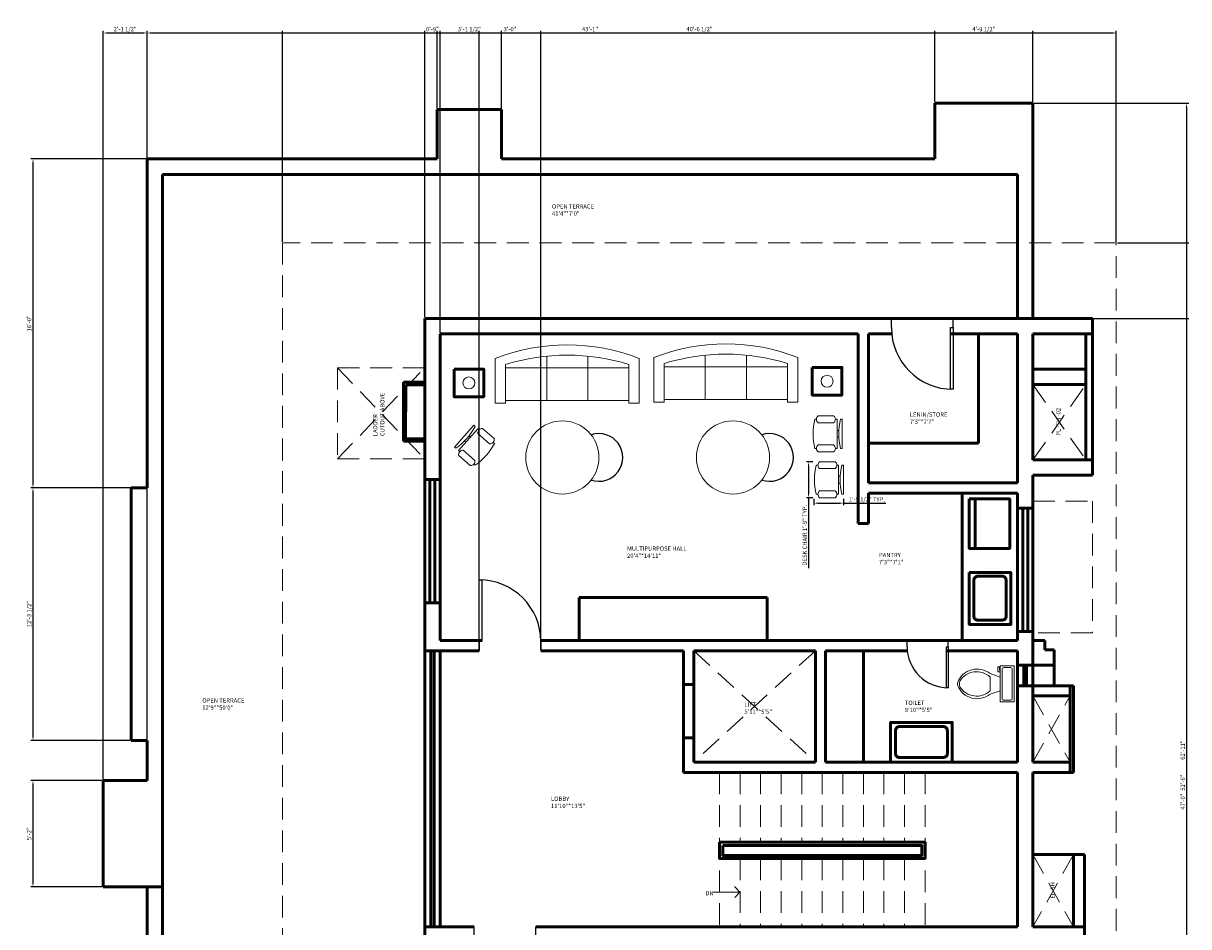
# Model space of a CAD drawing. Units: inches. Extents: x 5312 to 23584, y 2846 to 7447.
# Tile 8 of 12: x 10620 to 11300, y 3352 to 3879. Entities that reach past the tile are written whole.
import ezdxf

# ---------------------------------------------------------------- set-up
doc = ezdxf.new("R2010")
doc.units = ezdxf.units.IN
doc.linetypes.add('DASHED', pattern=[19.05, 12.7, -6.35])
for name, color, linetype, lineweight in [('A-ANNO-DIMS', 2, 'Continuous', 18), ('A-ANNO-TEXT', 3, 'Continuous', 18), ('A-AREA-IDEN', 7, 'Continuous', 18), ('A-DOOR', 4, 'Continuous', 25), ('A-FLOR-FIXT', 9, 'Continuous', 18), ('A-FLOR-OVHD', 8, 'DASHED', 18), ('A-FLOR-STRS', 3, 'Continuous', 18), ('A-FURN', 8, 'Continuous', 18), ('A-WALL', 7, 'Continuous', 50)]:
    doc.layers.add(name, color=color, linetype=linetype, lineweight=lineweight)
doc.styles.get("Standard").update_dxf_attribs({"font": 'arial.ttf'})
doc.dimstyles.new('ISO-25', dxfattribs={"dimtxt": 2.5, "dimasz": 2.5, "dimexe": 1.25, "dimexo": 0.625, "dimtad": 1, "dimlunit": 3, "dimtxsty": 'Standard', "dimcen": 2.5, "dimadec": 0, "dimazin": 0, "dimtfac": 1, "dimtmove": 0, "dimatfit": 3, "dimfxl": 1, "dimarcsym": 0})

# ---------------------------------------------------------------- blocks, each defined once
blk = doc.blocks.new('*U2')
for p, q in [((0, 0), (0, -6)), ((40, 0), (40, -6))]:
    blk.add_line(p, q)
blk.add_lwpolyline([(0, 0), (0, 40), (1.75, 40), (1.75, 0)], close=True)
blk.add_arc((0, 0), 40, 0, 90)
blk = doc.blocks.new('Sofa - Roundback 7 ft.')
for p, q in [((-12.00002, -32.4421), (-12.00003, -6.5971)), ((11.99997, -32.4421), (11.99998, -6.5971)), ((-36.000027, -34), (-36.000027, -11.4696)), ((-35.999844, -13.3819), (35.9998, -13.3819)), ((35.99998, -34), (35.99998, -11.4696)), ((-36.000027, -32.4421), (35.99998, -32.4421))]:
    blk.add_line(p, q)
for points in [[(-36.000027, -34), (-42.000027, -34), (-42.000027, -8)], [(41.99998, -8), (41.99998, -34), (35.99998, -34)]]:
    blk.add_lwpolyline(points)
for centre, radius, start, end in [((0, -114.25), 114.25, 68.43141, 111.5686), ((-0.00001, -127.1968), 121.1968, 72.72033, 107.2797)]:
    blk.add_arc(centre, radius, start, end)
blk = doc.blocks.new('Chair - Desk')
for p, q in [((-8.5, 0), (-8.5, -1)), ((-8.5, 0), (8.5, 0)), ((8.5, 0), (8.5, -1)), ((-10.5, -5), (-10.5, -14)), ((-8.5, -3), (-8.5, -4)), ((-8.5, -3), (8.5, -3)), ((-6.5, -14), (-6.5, -5)), ((-2, -3), (-2, -1.9355)), ((2, -1.9576), (2, -3)), ((6.5, -5), (6.5, -14)), ((8.5, -3), (8.5, -4)), ((10.5, -14), (10.5, -5)), ((-8.5, -15), (-8.5, -16)), ((8.5, -15), (8.5, -16))]:
    blk.add_line(p, q)
for centre, radius, start, end in [((-8.5, -6.5), 2.5, 36.8699, 143.1301), ((0, 34.625), 36.625, 256.5803, 283.4197), ((8.5, -6.5), 2.5, 36.8699, 143.1301), ((-8.5, -12.5), 2.5, 216.8699, 323.1301), ((0, 19.625), 36.625, 256.5803, 283.4197), ((8.5, -12.5), 2.5, 216.8699, 323.1301)]:
    blk.add_arc(centre, radius, start, end)
blk = doc.blocks.new('Toilet - top')
for p, q in [((9.5, -6), (9.5, -2)), ((-10, -8.5), (-8, -8.5)), ((-10, -9.5), (-10, -8.5)), ((-7, -9.5), (-10, -9.5)), ((-8, -8.5), (-8, -8)), ((-7, -8), (-7, -9.5)), ((-4, -8), (-6, -14)), ((4, -8), (6, -14)), ((4, -14), (-4, -14))]:
    blk.add_line(p, q)
blk.add_lwpolyline([(10.5, -8), (10.5, 0), (-10.5, 0), (-10.5, -8)], close=True)
for points in [[(-9.5, -2), (-9.5, -6)], [(8.5, -1), (-8.5, -1)], [(-8.5, -7), (8.5, -7)]]:
    blk.add_lwpolyline(points)
for centre, radius, start, end in [((-8.62, -1.88), 0.884, 81.8699, 188.1301), ((-8.62, -6.12), 0.884, 171.8699, 278.1301), ((8.62, -1.88), 0.884, 351.8699, 98.1301), ((8.62, -6.12), 0.884, 261.8699, 8.1301), ((3.52, -21.58), 12.17, 141.46911, 247.97143), ((4.2, -21.82), 11.33, 136.36773, 238.94682), ((-3.52, -21.58), 12.17, 292.02843, 38.53071), ((-4.2, -21.82), 11.33, 301.05301, 43.63209), ((0, -27.88), 4, 245.73182, 294.26817), ((0, -29), 4, 254.86053, 285.13947)]:
    blk.add_arc(centre, radius, start, end)
blk = doc.blocks.new('STAIR-ARROW')
for p, q in [((0, 3.17), (16.03, 3.17)), ((16.03, 3.17), (12.89, 6.38)), ((16.03, 3.17), (13.15, 0))]:
    blk.add_line(p, q)
blk = doc.blocks.new('*D31')
at = {"layer": 'A-ANNO-DIMS', "color": 0, "lineweight": -2, "transparency": 16777216}
for p, q in [((11080.5, 3623.27), (11076.72, 3623.27)), ((11077.97, 3620.77), (11077.97, 3604.77)), ((11080.5, 3602.27), (11076.72, 3602.27)), ((11077.97, 3602.27), (11077.97, 3561.09))]:
    blk.add_line(p, q, dxfattribs=at)
at = {"layer": 'A-ANNO-DIMS', "color": 0, "transparency": 16777216}
for points in [[(11077.56, 3620.77), (11078.39, 3620.77), (11077.97, 3623.27)], [(11077.56, 3604.77), (11078.39, 3604.77), (11077.97, 3602.27)]]:
    blk.add_solid(points, dxfattribs=at)
at = {"layer": 'DEFPOINTS', "color": 0, "transparency": 16777216}
for p in [(11081.12, 3623.27), (11077.97, 3602.27), (11081.12, 3602.27)]:
    blk.add_point(p, dxfattribs=at)
at = {"layer": 'A-ANNO-DIMS', "color": 0, "transparency": 16777216, "insert": (11076.06, 3580.43), "char_height": 2.5, "attachment_point": 5, "rotation": 90}
blk.add_mtext('DESK CHAIR 1\'-9" TYP.', dxfattribs=at)
blk = doc.blocks.new('*D32')
at = {"layer": 'A-ANNO-DIMS', "color": 0, "lineweight": -2, "transparency": 16777216}
for p, q in [((11081.12, 3601.65), (11081.12, 3597.87)), ((11083.62, 3599.12), (11095.96, 3599.12)), ((11098.46, 3601.65), (11098.46, 3597.87)), ((11098.46, 3599.12), (11123.04, 3599.12))]:
    blk.add_line(p, q, dxfattribs=at)
at = {"layer": 'A-ANNO-DIMS', "color": 0, "transparency": 16777216}
for points in [[(11083.62, 3599.54), (11083.62, 3598.71), (11081.12, 3599.12)], [(11095.96, 3599.54), (11095.96, 3598.71), (11098.46, 3599.12)]]:
    blk.add_solid(points, dxfattribs=at)
at = {"layer": 'DEFPOINTS', "color": 0, "transparency": 16777216}
for p in [(11081.12, 3602.27), (11098.46, 3602.27), (11098.46, 3599.12)]:
    blk.add_point(p, dxfattribs=at)
at = {"layer": 'A-ANNO-DIMS', "color": 0, "transparency": 16777216, "insert": (11112, 3601.04), "char_height": 2.5, "attachment_point": 5}
blk.add_mtext('1\'-5 1/2" TYP.', dxfattribs=at)
blk = doc.blocks.new('*D83')
at = {"layer": 'A-ANNO-DIMS', "color": 0, "lineweight": -2, "transparency": 16777216}
for p, q in [((10691.96, 3800.6), (10691.96, 3874.73)), ((10694.46, 3873.48), (11206.46, 3873.48)), ((11208.96, 3800.6), (11208.96, 3874.73))]:
    blk.add_line(p, q, dxfattribs=at)
at = {"layer": 'A-ANNO-DIMS', "color": 0, "transparency": 16777216}
for points in [[(10694.46, 3873.9), (10694.46, 3873.07), (10691.96, 3873.48)], [(11206.46, 3873.9), (11206.46, 3873.07), (11208.96, 3873.48)]]:
    blk.add_solid(points, dxfattribs=at)
at = {"layer": 'DEFPOINTS', "color": 0, "transparency": 16777216}
for p in [(11208.96, 3873.48), (10691.96, 3799.97), (11208.96, 3799.97)]:
    blk.add_point(p, dxfattribs=at)
at = {"layer": 'A-ANNO-DIMS', "color": 0, "transparency": 16777216, "insert": (10950.46, 3875.39), "char_height": 2.5, "attachment_point": 5}
blk.add_mtext('43\'-1"', dxfattribs=at)
blk = doc.blocks.new('*D84')
at = {"layer": 'A-ANNO-DIMS', "color": 0, "lineweight": -2, "transparency": 16777216}
for p, q in [((11209.58, 3832.48), (11299.83, 3832.48)), ((11298.58, 3829.98), (11298.58, 3080.08)), ((11209.58, 3077.58), (11299.83, 3077.58))]:
    blk.add_line(p, q, dxfattribs=at)
at = {"layer": 'A-ANNO-DIMS', "color": 0, "transparency": 16777216}
for points in [[(11298.16, 3829.98), (11298.99, 3829.98), (11298.58, 3832.48)], [(11298.16, 3080.08), (11298.99, 3080.08), (11298.58, 3077.58)]]:
    blk.add_solid(points, dxfattribs=at)
at = {"layer": 'DEFPOINTS', "color": 0, "transparency": 16777216}
for p in [(11208.96, 3832.48), (11208.96, 3077.58), (11298.58, 3077.58)]:
    blk.add_point(p, dxfattribs=at)
at = {"layer": 'A-ANNO-DIMS', "color": 0, "transparency": 16777216, "insert": (11296.68, 3455.03), "char_height": 2.5, "attachment_point": 5, "rotation": 90}
blk.add_mtext('62\'-11"', dxfattribs=at)
blk = doc.blocks.new('*D85')
at = {"layer": 'A-ANNO-DIMS', "color": 0, "lineweight": -2, "transparency": 16777216}
for p, q in [((10666.36, 3437.87), (10666.36, 3874.73)), ((10668.86, 3873.48), (10689.46, 3873.48)), ((10691.96, 3461.27), (10691.96, 3874.73))]:
    blk.add_line(p, q, dxfattribs=at)
at = {"layer": 'A-ANNO-DIMS', "color": 0, "transparency": 16777216}
for points in [[(10668.86, 3873.9), (10668.86, 3873.07), (10666.36, 3873.48)], [(10689.46, 3873.9), (10689.46, 3873.07), (10691.96, 3873.48)]]:
    blk.add_solid(points, dxfattribs=at)
at = {"layer": 'DEFPOINTS', "color": 0, "transparency": 16777216}
for p in [(10691.96, 3873.48), (10691.96, 3460.64), (10666.36, 3437.25)]:
    blk.add_point(p, dxfattribs=at)
at = {"layer": 'A-ANNO-DIMS', "color": 0, "transparency": 16777216, "insert": (10679.16, 3875.4), "char_height": 2.5, "attachment_point": 5}
blk.add_mtext('2\'-1 1/2"', dxfattribs=at)
blk = doc.blocks.new('*D86')
at = {"layer": 'A-ANNO-DIMS', "color": 0, "lineweight": -2, "transparency": 16777216}
for p, q in [((10691.33, 3799.97), (10624.11, 3799.97)), ((10625.36, 3797.47), (10625.36, 3610.55)), ((10691.33, 3608.05), (10624.11, 3608.05))]:
    blk.add_line(p, q, dxfattribs=at)
at = {"layer": 'A-ANNO-DIMS', "color": 0, "transparency": 16777216}
for points in [[(10624.94, 3797.47), (10625.78, 3797.47), (10625.36, 3799.97)], [(10624.94, 3610.55), (10625.78, 3610.55), (10625.36, 3608.05)]]:
    blk.add_solid(points, dxfattribs=at)
at = {"layer": 'DEFPOINTS', "color": 0, "transparency": 16777216}
for p in [(10691.96, 3799.97), (10625.36, 3608.05), (10691.96, 3608.05)]:
    blk.add_point(p, dxfattribs=at)
at = {"layer": 'A-ANNO-DIMS', "color": 0, "transparency": 16777216, "insert": (10623.46, 3704.01), "char_height": 2.5, "attachment_point": 5, "rotation": 90}
blk.add_mtext('16\'-0"', dxfattribs=at)
blk = doc.blocks.new('*D87')
at = {"layer": 'A-ANNO-DIMS', "color": 0, "lineweight": -2, "transparency": 16777216}
for p, q in [((10682.12, 3608.05), (10624.11, 3608.05)), ((10625.36, 3605.55), (10625.36, 3463.14)), ((10682.12, 3460.64), (10624.11, 3460.64))]:
    blk.add_line(p, q, dxfattribs=at)
at = {"layer": 'A-ANNO-DIMS', "color": 0, "transparency": 16777216}
for points in [[(10624.94, 3605.55), (10625.78, 3605.55), (10625.36, 3608.05)], [(10624.94, 3463.14), (10625.78, 3463.14), (10625.36, 3460.64)]]:
    blk.add_solid(points, dxfattribs=at)
at = {"layer": 'DEFPOINTS', "color": 0, "transparency": 16777216}
for p in [(10682.74, 3608.05), (10625.36, 3460.64), (10682.74, 3460.64)]:
    blk.add_point(p, dxfattribs=at)
at = {"layer": 'A-ANNO-DIMS', "color": 0, "transparency": 16777216, "insert": (10623.44, 3534.35), "char_height": 2.5, "attachment_point": 5, "rotation": 90}
blk.add_mtext('12\'-3 1/2"', dxfattribs=at)
blk = doc.blocks.new('*D88')
at = {"layer": 'A-ANNO-DIMS', "color": 0, "lineweight": -2, "transparency": 16777216}
for p, q in [((10665.73, 3437.25), (10624.11, 3437.25)), ((10625.36, 3434.75), (10625.36, 3377.7)), ((10665.73, 3375.2), (10624.11, 3375.2))]:
    blk.add_line(p, q, dxfattribs=at)
at = {"layer": 'A-ANNO-DIMS', "color": 0, "transparency": 16777216}
for points in [[(10624.94, 3434.75), (10625.78, 3434.75), (10625.36, 3437.25)], [(10624.94, 3377.7), (10625.78, 3377.7), (10625.36, 3375.2)]]:
    blk.add_solid(points, dxfattribs=at)
at = {"layer": 'DEFPOINTS', "color": 0, "transparency": 16777216}
for p in [(10666.36, 3437.25), (10625.36, 3375.2), (10666.36, 3375.2)]:
    blk.add_point(p, dxfattribs=at)
at = {"layer": 'A-ANNO-DIMS', "color": 0, "transparency": 16777216, "insert": (10623.46, 3406.22), "char_height": 2.5, "attachment_point": 5, "rotation": 90}
blk.add_mtext('5\'-2"', dxfattribs=at)
blk = doc.blocks.new('*D91')
at = {"layer": 'A-ANNO-DIMS', "color": 0, "lineweight": -2, "transparency": 16777216}
for p, q in [((11200.58, 3706.97), (11299.83, 3706.97)), ((11298.58, 3704.47), (11298.58, 3145.47)), ((11200.58, 3142.97), (11299.83, 3142.97))]:
    blk.add_line(p, q, dxfattribs=at)
at = {"layer": 'A-ANNO-DIMS', "color": 0, "transparency": 16777216}
for points in [[(11298.16, 3704.47), (11298.99, 3704.47), (11298.58, 3706.97)], [(11298.16, 3145.47), (11298.99, 3145.47), (11298.58, 3142.97)]]:
    blk.add_solid(points, dxfattribs=at)
at = {"layer": 'DEFPOINTS', "color": 0, "transparency": 16777216}
for p in [(11199.96, 3706.97), (11199.96, 3142.97), (11298.58, 3142.97)]:
    blk.add_point(p, dxfattribs=at)
at = {"layer": 'A-ANNO-DIMS', "color": 0, "transparency": 16777216, "insert": (11296.68, 3424.97), "char_height": 2.5, "attachment_point": 5, "rotation": 90}
blk.add_mtext('47\'-0"', dxfattribs=at)
blk = doc.blocks.new('*D92')
at = {"layer": 'A-ANNO-DIMS', "color": 0, "lineweight": -2, "transparency": 16777216}
for p, q in [((10861.16, 3829.39), (10861.16, 3874.73)), ((10863.66, 3873.48), (10896.32, 3873.48)), ((10898.82, 3829.39), (10898.82, 3874.73))]:
    blk.add_line(p, q, dxfattribs=at)
at = {"layer": 'A-ANNO-DIMS', "color": 0, "transparency": 16777216}
for points in [[(10863.66, 3873.9), (10863.66, 3873.07), (10861.16, 3873.48)], [(10896.32, 3873.9), (10896.32, 3873.07), (10898.82, 3873.48)]]:
    blk.add_solid(points, dxfattribs=at)
at = {"layer": 'DEFPOINTS', "color": 0, "transparency": 16777216}
for p in [(10898.82, 3873.48), (10861.16, 3828.76), (10898.82, 3828.76)]:
    blk.add_point(p, dxfattribs=at)
at = {"layer": 'A-ANNO-DIMS', "color": 0, "transparency": 16777216, "insert": (10879.99, 3875.4), "char_height": 2.5, "attachment_point": 5}
blk.add_mtext('3\'-1 1/2"', dxfattribs=at)
blk = doc.blocks.new('*D93')
at = {"layer": 'A-ANNO-DIMS', "color": 0, "lineweight": -2, "transparency": 16777216}
for p, q in [((11151.61, 3833.11), (11151.61, 3874.73)), ((11154.11, 3873.48), (11206.46, 3873.48)), ((11208.96, 3833.11), (11208.96, 3874.73))]:
    blk.add_line(p, q, dxfattribs=at)
at = {"layer": 'A-ANNO-DIMS', "color": 0, "transparency": 16777216}
for points in [[(11154.11, 3873.9), (11154.11, 3873.07), (11151.61, 3873.48)], [(11206.46, 3873.9), (11206.46, 3873.07), (11208.96, 3873.48)]]:
    blk.add_solid(points, dxfattribs=at)
at = {"layer": 'DEFPOINTS', "color": 0, "transparency": 16777216}
for p in [(11208.96, 3873.48), (11151.61, 3832.48), (11208.96, 3832.48)]:
    blk.add_point(p, dxfattribs=at)
at = {"layer": 'A-ANNO-DIMS', "color": 0, "transparency": 16777216, "insert": (11180.28, 3875.4), "char_height": 2.5, "attachment_point": 5}
blk.add_mtext('4\'-9 1/2"', dxfattribs=at)
blk = doc.blocks.new('*D94')
at = {"layer": 'A-ANNO-DIMS', "color": 0, "lineweight": -2, "transparency": 16777216}
for p, q in [((10771.06, 3751.69), (10771.06, 3874.73)), ((10773.56, 3873.48), (11255.08, 3873.48)), ((11257.58, 3751.69), (11257.58, 3874.73))]:
    blk.add_line(p, q, dxfattribs=at)
at = {"layer": 'A-ANNO-DIMS', "color": 0, "transparency": 16777216}
for points in [[(10773.56, 3873.9), (10773.56, 3873.07), (10771.06, 3873.48)], [(11255.08, 3873.9), (11255.08, 3873.07), (11257.58, 3873.48)]]:
    blk.add_solid(points, dxfattribs=at)
at = {"layer": 'DEFPOINTS', "color": 0, "transparency": 16777216}
for p in [(11257.58, 3873.48), (10771.06, 3751.07), (11257.58, 3751.07)]:
    blk.add_point(p, dxfattribs=at)
at = {"layer": 'A-ANNO-DIMS', "color": 0, "transparency": 16777216, "insert": (11014.32, 3875.4), "char_height": 2.5, "attachment_point": 5}
blk.add_mtext('40\'-6 1/2"', dxfattribs=at)
blk = doc.blocks.new('*D95')
at = {"layer": 'A-ANNO-DIMS', "color": 0, "lineweight": -2, "transparency": 16777216}
for p, q in [((11258.2, 3751.07), (11299.83, 3751.07)), ((11298.58, 3748.57), (11298.58, 3123.52)), ((11258.2, 3121.02), (11299.83, 3121.02))]:
    blk.add_line(p, q, dxfattribs=at)
at = {"layer": 'A-ANNO-DIMS', "color": 0, "transparency": 16777216}
for points in [[(11298.16, 3748.57), (11298.99, 3748.57), (11298.58, 3751.07)], [(11298.16, 3123.52), (11298.99, 3123.52), (11298.58, 3121.02)]]:
    blk.add_solid(points, dxfattribs=at)
at = {"layer": 'DEFPOINTS', "color": 0, "transparency": 16777216}
for p in [(11257.58, 3751.07), (11257.58, 3121.02), (11298.58, 3121.02)]:
    blk.add_point(p, dxfattribs=at)
at = {"layer": 'A-ANNO-DIMS', "color": 0, "transparency": 16777216, "insert": (11296.68, 3436.04), "char_height": 2.5, "attachment_point": 5, "rotation": 90}
blk.add_mtext('52\'-6"', dxfattribs=at)
blk = doc.blocks.new('*D96')
at = {"layer": 'A-ANNO-DIMS', "color": 0, "lineweight": -2, "transparency": 16777216}
for p, q in [((10853.96, 3707.6), (10853.96, 3874.73)), ((10856.46, 3873.48), (10860.46, 3873.48)), ((10862.96, 3698.6), (10862.96, 3874.73))]:
    blk.add_line(p, q, dxfattribs=at)
at = {"layer": 'A-ANNO-DIMS', "color": 0, "transparency": 16777216}
for points in [[(10856.46, 3873.9), (10856.46, 3873.07), (10853.96, 3873.48)], [(10860.46, 3873.9), (10860.46, 3873.07), (10862.96, 3873.48)]]:
    blk.add_solid(points, dxfattribs=at)
at = {"layer": 'DEFPOINTS', "color": 0, "transparency": 16777216}
for p in [(10862.96, 3873.48), (10853.96, 3706.97), (10862.96, 3697.97)]:
    blk.add_point(p, dxfattribs=at)
at = {"layer": 'A-ANNO-DIMS', "color": 0, "transparency": 16777216, "insert": (10858.46, 3875.39), "char_height": 2.5, "attachment_point": 5}
blk.add_mtext('0\'-9"', dxfattribs=at)
blk = doc.blocks.new('*D98')
at = {"layer": 'A-ANNO-DIMS', "color": 0, "lineweight": -2, "transparency": 16777216}
for p, q in [((10885.75, 3513.6), (10885.75, 3874.73)), ((10888.25, 3873.48), (10919.25, 3873.48)), ((10921.75, 3513.6), (10921.75, 3874.73))]:
    blk.add_line(p, q, dxfattribs=at)
at = {"layer": 'A-ANNO-DIMS', "color": 0, "transparency": 16777216}
for points in [[(10888.25, 3873.9), (10888.25, 3873.07), (10885.75, 3873.48)], [(10919.25, 3873.9), (10919.25, 3873.07), (10921.75, 3873.48)]]:
    blk.add_solid(points, dxfattribs=at)
at = {"layer": 'DEFPOINTS', "color": 0, "transparency": 16777216}
for p in [(10921.75, 3873.48), (10885.75, 3512.97), (10921.75, 3512.97)]:
    blk.add_point(p, dxfattribs=at)
at = {"layer": 'A-ANNO-DIMS', "color": 0, "transparency": 16777216, "insert": (10903.75, 3875.39), "char_height": 2.5, "attachment_point": 5}
blk.add_mtext('3\'-0"', dxfattribs=at)

msp = doc.modelspace()

# ---------------------------------------------------------------- linework, layer by layer
at = {"layer": 'A-DOOR'}
for centre in [(10955.653, 3625.785), (11055.243, 3625.785)]:
    msp.add_arc(centre, 13.919, 250.983481, 109.016519, dxfattribs=at)
at = {"layer": 'A-FLOR-OVHD'}
for p, q in [((10771.06, 3751.067), (10771.06, 3121.017)), ((11257.577, 3751.067), (10771.06, 3751.067)), ((11257.577, 3121.017), (11257.577, 3751.067)), ((10853.956, 3678.136), (10803.054, 3678.136)), ((10803.054, 3678.136), (10803.054, 3624.911)), ((10803.054, 3678.136), (10853.956, 3624.911)), ((10803.054, 3624.911), (10853.956, 3678.136)), ((11208.956, 3668.309), (11239.801, 3624.391)), ((11208.956, 3624.391), (11239.801, 3668.309)), ((10803.054, 3624.911), (10853.956, 3624.911)), ((10803.054, 3624.911), (10803.054, 3624.911)), ((11208.956, 3600.303), (11243.661, 3600.303)), ((11243.661, 3600.303), (11243.661, 3523.522)), ((11243.661, 3523.522), (11208.956, 3523.522)), ((11010.956, 3512.971), (11081.956, 3447.971)), ((11081.956, 3512.971), (11010.956, 3447.971)), ((11208.956, 3486.615), (11230.578, 3447.971)), ((11208.956, 3447.971), (11230.578, 3486.615)), ((11025.998, 3441.971), (11025.998, 3351.971)), ((11037.998, 3441.971), (11037.998, 3401.281)), ((11049.998, 3441.971), (11049.998, 3401.281)), ((11061.998, 3441.971), (11061.998, 3401.281)), ((11073.998, 3441.971), (11073.998, 3401.281)), ((11085.998, 3441.971), (11085.998, 3401.281)), ((11097.998, 3441.971), (11097.998, 3401.281)), ((11109.998, 3441.971), (11109.998, 3401.281)), ((11121.998, 3441.971), (11121.998, 3401.281)), ((11133.998, 3441.971), (11133.998, 3401.281)), ((11145.998, 3441.971), (11145.998, 3351.971)), ((11208.956, 3394.056), (11232.596, 3351.971)), ((11232.596, 3394.056), (11208.956, 3351.971)), ((11037.998, 3391.78), (11037.998, 3351.971)), ((11049.998, 3391.78), (11049.998, 3351.971)), ((11061.998, 3391.78), (11061.998, 3351.971)), ((11073.998, 3391.78), (11073.998, 3351.971)), ((11085.998, 3391.78), (11085.998, 3351.971)), ((11097.998, 3391.78), (11097.998, 3351.971)), ((11109.998, 3391.78), (11109.998, 3351.971)), ((11121.998, 3391.78), (11121.998, 3351.971)), ((11133.998, 3391.78), (11133.998, 3351.971))]:
    msp.add_line(p, q, dxfattribs=at)
at = {"layer": 'A-FURN'}
for centre, radius in [((10879.743, 3669.29), 3.486), ((11088.82, 3670.277), 3.486), ((10934.294, 3625.785), 21.359), ((11033.884, 3625.785), 21.359)]:
    msp.add_circle(centre, radius, dxfattribs=at)
at = {"layer": 'A-WALL'}
for p, q in [((11208.956, 3832.484), (11151.608, 3832.484)), ((11151.608, 3832.484), (11151.608, 3799.971)), ((11208.956, 3799.971), (11208.956, 3832.484)), ((10898.825, 3828.763), (10861.161, 3828.763)), ((10861.161, 3828.763), (10861.161, 3799.971)), ((10898.825, 3799.971), (10898.825, 3828.763)), ((10691.956, 3799.971), (10861.161, 3799.971)), ((10691.956, 3608.047), (10691.956, 3799.971)), ((10898.825, 3799.971), (11151.608, 3799.971)), ((11208.956, 3706.971), (11208.956, 3799.971)), ((10700.956, 3790.971), (10700.956, 3108.64)), ((10700.956, 3790.971), (11199.956, 3790.971)), ((11199.956, 3790.971), (11199.956, 3706.971)), ((10853.956, 3706.971), (10853.956, 3142.971)), ((10853.956, 3706.971), (11208.956, 3706.971)), ((11208.956, 3706.971), (11239.801, 3706.971)), ((11239.801, 3706.971), (11243.661, 3706.971)), ((11243.661, 3706.971), (11243.661, 3615.391)), ((10862.956, 3697.971), (10862.956, 3518.971)), ((10862.956, 3697.971), (11106.956, 3697.971)), ((11106.956, 3697.971), (11106.956, 3587.288)), ((11112.956, 3697.971), (11112.956, 3610.971)), ((11112.956, 3697.971), (11126.484, 3697.971)), ((11160.728, 3697.971), (11199.956, 3697.971)), ((11177.225, 3634.083), (11177.225, 3697.971)), ((11199.956, 3697.971), (11199.956, 3610.971)), ((11208.956, 3697.971), (11208.956, 3624.391)), ((11243.661, 3697.971), (11208.956, 3697.971)), ((11239.801, 3697.971), (11239.801, 3677.309)), ((11208.956, 3677.309), (11239.801, 3677.309)), ((11239.801, 3677.309), (11239.801, 3668.309)), ((10853.956, 3669.775), (10841.635, 3669.775)), ((10841.635, 3669.775), (10841.635, 3635.234)), ((10842.979, 3668.129), (10842.674, 3636.708)), ((10853.956, 3668.129), (10842.979, 3668.129)), ((11208.956, 3668.309), (11239.801, 3668.309)), ((11239.801, 3668.309), (11239.801, 3624.391)), ((10841.635, 3635.234), (10853.956, 3635.234)), ((10842.674, 3636.708), (10853.956, 3636.708)), ((11112.956, 3634.083), (11177.225, 3634.083)), ((11208.956, 3624.391), (11243.661, 3624.391)), ((10853.956, 3540.882), (10853.956, 3612.882)), ((10853.956, 3612.882), (10862.956, 3612.882)), ((10856.956, 3540.882), (10856.956, 3612.882)), ((10859.956, 3612.882), (10859.956, 3540.882)), ((10862.956, 3612.882), (10862.956, 3540.882)), ((11208.956, 3615.391), (11239.801, 3615.391)), ((11208.956, 3615.391), (11208.956, 3447.971)), ((11243.661, 3615.391), (11239.801, 3615.391)), ((10682.741, 3460.645), (10682.741, 3608.047)), ((10682.741, 3608.047), (10691.956, 3608.047)), ((11112.956, 3610.971), (11199.956, 3610.971)), ((11112.956, 3604.971), (11199.956, 3604.971)), ((11112.956, 3604.971), (11112.956, 3587.288)), ((11167.712, 3604.971), (11167.712, 3604.113)), ((11199.956, 3604.971), (11199.956, 3518.971)), ((11167.712, 3604.113), (11167.712, 3518.971)), ((11175.26, 3601.59), (11175.26, 3572.71)), ((11199.956, 3524.293), (11199.956, 3596.293)), ((11199.956, 3596.293), (11208.956, 3596.293)), ((11202.956, 3524.293), (11202.956, 3596.293)), ((11205.956, 3596.293), (11205.956, 3524.293)), ((11208.956, 3596.293), (11208.956, 3524.293)), ((11106.956, 3587.288), (11112.956, 3587.288)), ((10944.154, 3520.543), (10944.154, 3543.97)), ((10944.154, 3543.97), (11053.898, 3543.97)), ((11053.898, 3543.97), (11053.898, 3518.971)), ((10862.956, 3540.882), (10853.956, 3540.882)), ((11208.956, 3524.293), (11199.956, 3524.293)), ((10862.956, 3518.971), (10887.329, 3518.971)), ((10921.749, 3518.971), (11106.956, 3518.971)), ((10944.154, 3518.971), (10944.154, 3520.543)), ((11053.898, 3518.971), (11199.956, 3518.971)), ((11208.956, 3518.971), (11215.783, 3518.971)), ((11215.783, 3518.971), (11215.783, 3513.556)), ((10853.956, 3512.971), (10885.754, 3512.971)), ((10857.536, 3512.971), (10857.536, 3351.971)), ((10859.394, 3512.971), (10859.394, 3351.971)), ((10862.956, 3512.971), (10862.956, 3351.971)), ((10921.754, 3512.971), (11004.956, 3512.971)), ((11004.956, 3512.971), (11004.956, 3441.971)), ((11010.956, 3512.971), (11010.956, 3447.971)), ((11010.956, 3512.971), (11081.956, 3512.971)), ((11081.956, 3512.971), (11081.956, 3447.971)), ((11087.956, 3512.971), (11087.956, 3447.971)), ((11087.956, 3512.971), (11135.622, 3512.971)), ((11109.959, 3512.971), (11109.959, 3447.971)), ((11158.452, 3512.971), (11199.956, 3512.971)), ((11199.956, 3512.971), (11199.956, 3447.971)), ((11215.783, 3513.556), (11221.343, 3513.556)), ((11221.343, 3513.556), (11221.343, 3492.615)), ((11199.956, 3504.556), (11221.343, 3504.556)), ((11203.6, 3504.556), (11203.6, 3492.615)), ((11205.101, 3504.556), (11205.101, 3492.615)), ((11004.956, 3493.217), (11010.956, 3493.217)), ((11221.163, 3492.615), (11199.956, 3492.615)), ((11221.343, 3492.615), (11221.163, 3492.615)), ((11221.343, 3492.615), (11230.578, 3492.615)), ((11230.578, 3492.615), (11230.578, 3441.971)), ((11230.578, 3492.615), (11232.596, 3492.615)), ((11232.596, 3492.615), (11232.596, 3441.971)), ((11208.956, 3486.615), (11230.578, 3486.615)), ((11004.956, 3462.148), (11004.956, 3462.148)), ((11004.956, 3462.148), (11010.956, 3462.148)), ((10691.956, 3460.645), (10682.741, 3460.645)), ((10691.956, 3460.645), (10691.956, 3437.249)), ((11004.956, 3441.971), (11199.956, 3441.971)), ((11010.956, 3447.971), (11081.956, 3447.971)), ((11087.956, 3447.971), (11199.956, 3447.971)), ((11199.956, 3441.971), (11199.956, 3351.971)), ((11208.956, 3447.971), (11230.578, 3447.971)), ((11208.956, 3441.971), (11230.578, 3441.971)), ((11208.956, 3441.971), (11208.956, 3351.971)), ((11232.596, 3441.971), (11230.578, 3441.971)), ((10666.359, 3375.201), (10666.359, 3437.249)), ((10666.359, 3437.249), (10691.956, 3437.249)), ((11208.956, 3394.056), (11232.596, 3394.056)), ((11232.596, 3394.056), (11232.596, 3351.971)), ((11232.596, 3394.056), (11239.069, 3394.056)), ((11239.069, 3394.056), (11239.069, 3307.569)), ((10700.956, 3375.201), (10666.359, 3375.201)), ((10691.956, 3375.201), (10691.956, 3099.64)), ((10853.956, 3351.971), (10882.843, 3351.971)), ((10859.394, 3351.971), (10859.394, 3351.971)), ((10918.843, 3351.971), (11199.956, 3351.971)), ((11208.956, 3351.971), (11239.069, 3351.971))]:
    msp.add_line(p, q, dxfattribs=at)
for points in [[(10871.085, 3677.389), (10888.401, 3677.389), (10888.401, 3661.191), (10871.085, 3661.191)], [(11080.162, 3678.376), (11097.478, 3678.376), (11097.478, 3662.178), (11080.162, 3662.178)], [(11171.764, 3601.59), (11195.412, 3601.59), (11195.412, 3572.71), (11171.764, 3572.71)], [(11171.764, 3558.63), (11196.044, 3558.63), (11196.044, 3528.326), (11171.764, 3528.326)], [(11125.887, 3447.971), (11161.8, 3447.971), (11161.8, 3471.19), (11125.887, 3471.19)], [(11025.998, 3401.281), (11145.998, 3401.281), (11145.998, 3391.78), (11025.998, 3391.78)], [(11027.889, 3399.318), (11144.176, 3399.318), (11144.176, 3393.606), (11027.889, 3393.606)]]:
    msp.add_lwpolyline(points, close=True, dxfattribs=at)
for points in [[(11176.93, 3556.559), (11190.863, 3556.559, -0.4142136), (11193.363, 3554.059), (11193.363, 3533.261, -0.4142136), (11190.863, 3530.761), (11176.93, 3530.761, -0.4142136), (11174.43, 3533.261), (11174.43, 3554.059, -0.4142136)], [(11131.145, 3468.757), (11156.516, 3468.757, -0.4142136), (11159.016, 3466.257), (11159.016, 3453.12, -0.4142136), (11156.516, 3450.62), (11131.145, 3450.62, -0.4142136), (11128.645, 3453.12), (11128.645, 3466.257, -0.4142136)]]:
    msp.add_lwpolyline(points, format="xyb", close=True, dxfattribs=at)

# ---------------------------------------------------------------- block references
at = {"layer": 'A-DOOR', "rotation": 180}
for p, xscale, yscale, zscale in [((11162.303, 3701.571), 0.9, 0.9, 0.9), ((11159.502, 3515.371), 0.6, 0.6, 0.6), ((10882.843, 3346.571), -0.9, 0.9, 0.9)]:
    msp.add_blockref('*U2', p, dxfattribs=dict(at, xscale=xscale, yscale=yscale, zscale=zscale))
at = {"layer": 'A-DOOR', "xscale": 0.9, "yscale": 0.9, "zscale": 0.9}
msp.add_blockref('*U2', (10885.754, 3518.371), dxfattribs=at)
at = {"layer": 'A-FLOR-FIXT', "rotation": 270}
msp.add_blockref('Toilet - top', (11197.877, 3493.638), dxfattribs=at)
at = {"layer": 'A-FLOR-STRS', "rotation": 359.7532758824103}
msp.add_blockref('STAIR-ARROW', (11021.842, 3369.04), dxfattribs=at)
at = {"layer": 'A-FURN'}
for p in [(10937.169, 3691.509), (11029.724, 3692.079)]:
    msp.add_blockref('Sofa - Roundback 7 ft.', p, dxfattribs=at)
for p, rotation in [((10877.015, 3638.168), 48.50241121697704), ((11097.622, 3639.562), 270), ((11098.458, 3612.774), 270)]:
    msp.add_blockref('Chair - Desk', p, dxfattribs=dict(at, rotation=rotation))

# ---------------------------------------------------------------- texts
at = {"layer": 'A-ANNO-TEXT', "char_height": 2.5, "attachment_point": 1, "rotation": 90}
for s, width, insert in [('PL -SH -02', 22.22169, (11222.537, 3638.49)), ('EL-SH', 15.51135, (11219.191, 3368.376))]:
    msp.add_mtext_dynamic_manual_height_columns(s, width=width, gutter_width=12.5, heights=[0], dxfattribs=dict(at, insert=insert))
at = {"layer": 'A-ANNO-TEXT', "insert": (11017.782, 3372.694), "char_height": 2.5, "attachment_point": 1}
msp.add_mtext_dynamic_manual_height_columns('DN', width=4.55078, gutter_width=12.5, heights=[0], dxfattribs=at)
at = {"layer": 'A-AREA-IDEN', "char_height": 2.5, "attachment_point": 1}
for s, width, insert in [('OPEN TERRACE\\P41\'4"*7\'0"', 87.24423, (10928.218, 3773.556)), ('LENIN/STORE\\P7\'3"*7\'7"', 45.60856, (11137.101, 3652.061)), ('MULTIPURPOSE HALL\\P20\'4"*14\'11"', 121.00985, (10972.069, 3573.871)), ('PANTRY\\P7\'3"*7\'1"', 40.55875, (11119.088, 3570.118)), ('OPEN TERRACE\\P12\'9"*50\'0"', 51.00783, (10724.173, 3485.231)), ('LIFT\\P5\'11"*5\'5"', 42.62605, (11040.521, 3482.851)), ('TOILET\\P8\'10"*5\'5"', 43.70587, (11134.175, 3483.868)), ('LOBBY\\P11\'10"*13\'5"', 80.64925, (10927.661, 3427.859))]:
    msp.add_mtext_dynamic_manual_height_columns(s, width=width, gutter_width=12.5, heights=[0], dxfattribs=dict(at, insert=insert))
at = {"layer": 'A-AREA-IDEN', "insert": (10823.823, 3638.256), "char_height": 2.5, "attachment_point": 1, "rotation": 90}
msp.add_mtext_dynamic_manual_height_columns('LADDER\\PCUTOUT ABOVE', width=28.25938, gutter_width=12.5, heights=[0], dxfattribs=at)

# ---------------------------------------------------------------- dimensions: what is measured, and where the dimension line sits
at = {"layer": 'A-ANNO-DIMS'}
for base, p1, p2, picture, middle in [((10691.956, 3873.484), (10666.359, 3437.249), (10691.956, 3460.645), '*D85', (10679.158, 3875.402)), ((11208.956, 3873.484), (10691.956, 3799.971), (11208.956, 3799.971), '*D83', (10950.456, 3875.387)), ((11257.577, 3873.484), (10771.06, 3751.067), (11257.577, 3751.067), '*D94', (11014.319, 3875.402)), ((10862.956, 3873.484), (10853.956, 3706.971), (10862.956, 3697.971), '*D96', (10858.456, 3875.386)), ((10898.825, 3873.484), (10861.161, 3828.763), (10898.825, 3828.763), '*D92', (10879.993, 3875.403)), ((10921.754, 3873.484), (10885.754, 3512.971), (10921.754, 3512.971), '*D98', (10903.754, 3875.387)), ((11208.956, 3873.484), (11151.608, 3832.484), (11208.956, 3832.484), '*D93', (11180.282, 3875.402))]:
    dim = msp.add_linear_dim(base=base, p1=p1, p2=p2, dimstyle='ISO-25', override={"dimdec": 1, "dimlfac": 1, "dimrnd": 0, "dimzin": 1, "dimdsep": 46, "dimlunit": 4, "dimfrac": 2}, dxfattribs=at)
    dim.commit()
    dim.dimension.update_dxf_attribs({"geometry": picture, "text_midpoint": middle})
for base, p1, p2, picture, middle in [((11298.577, 3077.583), (11208.956, 3832.484), (11208.956, 3077.583), '*D84', (11296.675, 3455.034)), ((10625.359, 3608.047), (10691.956, 3799.971), (10691.956, 3608.047), '*D86', (10623.457, 3704.009)), ((11298.5767, 3121.0171), (11257.5767, 3751.0665), (11257.5767, 3121.0171), '*D95', (11296.6753, 3436.0418)), ((11298.577, 3142.971), (11199.956, 3706.971), (11199.956, 3142.971), '*D91', (11296.675, 3424.971)), ((10625.359, 3460.645), (10682.741, 3608.047), (10682.741, 3460.645), '*D87', (10623.44, 3534.346)), ((10625.359, 3375.201), (10666.359, 3437.249), (10666.359, 3375.201), '*D88', (10623.457, 3406.225))]:
    dim = msp.add_linear_dim(base=base, p1=p1, p2=p2, angle=90, dimstyle='ISO-25', override={"dimdec": 1, "dimlfac": 1, "dimrnd": 0, "dimzin": 1, "dimdsep": 46, "dimlunit": 4, "dimfrac": 2}, dxfattribs=at)
    dim.commit()
    dim.dimension.update_dxf_attribs({"geometry": picture, "text_midpoint": middle})
dim = msp.add_linear_dim(base=(11077.974, 3602.274), p1=(11081.124, 3623.274), p2=(11081.124, 3602.274), angle=270, text='DESK CHAIR <> TYP.', dimstyle='ISO-25', override={"dimdec": 1, "dimrnd": 0, "dimzin": 1, "dimlunit": 4, "dimfrac": 2}, dxfattribs=at)
dim.commit()
dim.dimension.update_dxf_attribs({"geometry": '*D31', "text_midpoint": (11076.057, 3580.433)})
dim = msp.add_linear_dim(base=(11098.458, 3599.124), p1=(11081.124, 3602.274), p2=(11098.458, 3602.274), text='<> TYP.', dimstyle='ISO-25', override={"dimdec": 1, "dimrnd": 0, "dimzin": 1, "dimlunit": 4, "dimfrac": 2}, dxfattribs=at)
dim.commit()
dim.dimension.update_dxf_attribs({"geometry": '*D32', "text_midpoint": (11111.997, 3601.041)})

doc.saveas('drawing.dxf')
